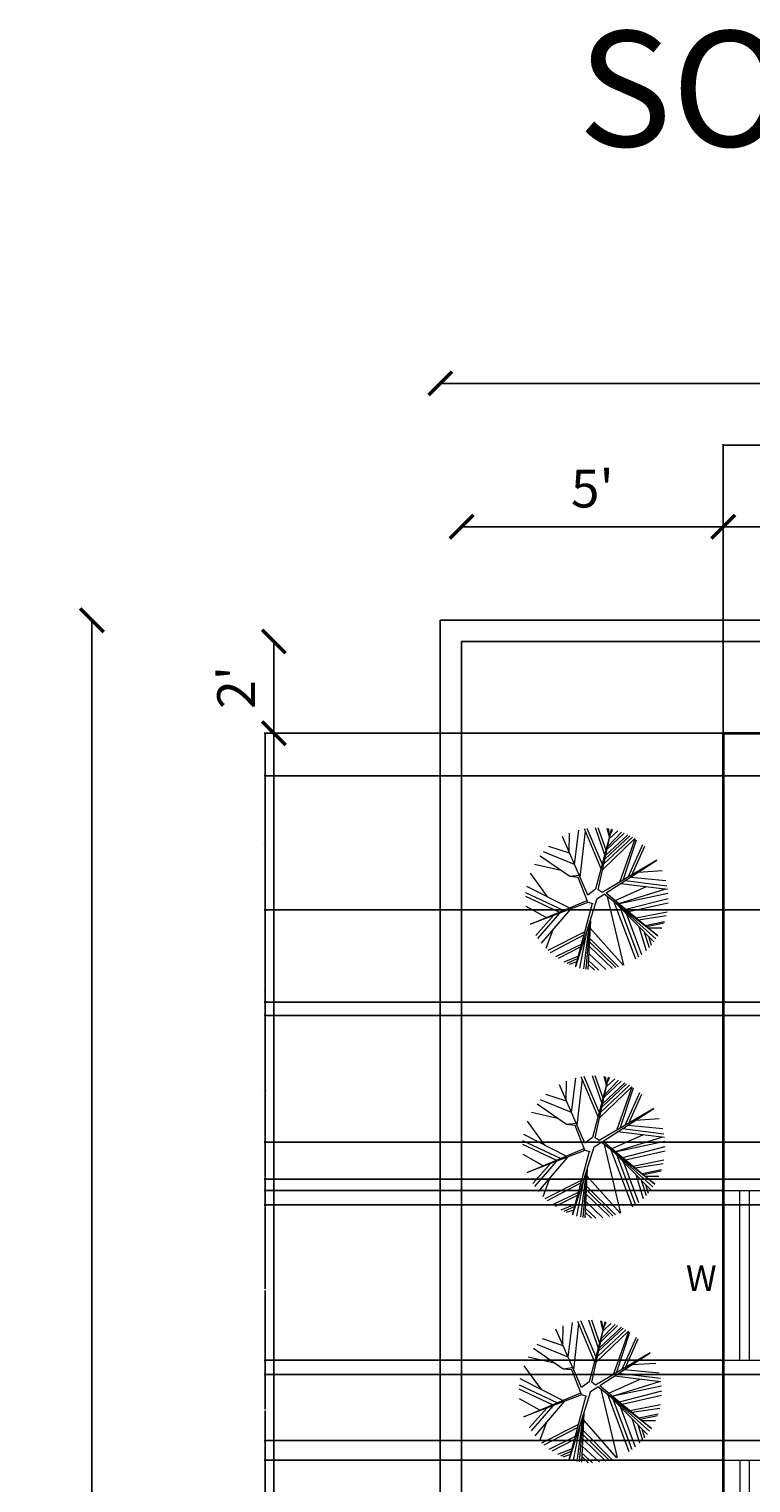
# Model space of a CAD drawing. Units: inches. Extents: x 503 to 1084, y -605 to 132.
# Tile 12 of 14: x 503 to 656, y -177 to 132. Entities that reach past the tile are written whole.
import ezdxf

# ---------------------------------------------------------------- set-up
doc = ezdxf.new("R2010")
doc.units = ezdxf.units.IN
doc.header["$MEASUREMENT"] = 0
for name, color, linetype, lineweight in [('A-ANNO-DIMS', 7, 'Continuous', 18), ('A-ANNO-TEXT', 7, 'Continuous', 18), ('C-PROP', 1, 'Continuous', 25), ('wall', 1, 'Continuous', 35), ('wind', 5, 'Continuous', 18)]:
    doc.layers.add(name, color=color, linetype=linetype, lineweight=lineweight)
doc.layers.add('GRASS', color=90, linetype='Continuous', lineweight=13, transparency=0.7)
doc.styles.get("Standard").update_dxf_attribs({"font": 'arial.ttf'})
doc.dimstyles.get("Standard").update_dxf_attribs({"dimtxt": 0.18, "dimasz": 0.18, "dimexe": 0.18, "dimexo": 0.0625, "dimgap": 0.09, "dimtad": 0, "dimtih": 1, "dimtoh": 1, "dimdec": 1, "dimzin": 0, "dimdsep": 46, "dimlunit": 4, "dimtxsty": 'Standard', "dimcen": 0.09, "dimadec": 0, "dimazin": 0, "dimtfac": 1, "dimtdec": 1, "dimtofl": 0, "dimtmove": 0, "dimatfit": 3, "dimfxl": 1, "dimtolj": 1, "dimtzin": 0, "dimarcsym": 0})

# ---------------------------------------------------------------- blocks, each defined once
blk = doc.blocks.new('A$C4FA53466')
at = {"color": 0}
for p, q in [((0.717, 0.864), (0.422, 1.538)), ((0.501, 1.356), (0.505, 1.578)), ((0.563, 1.216), (0.612, 1.614)), ((0.627, 1.07), (0.687, 1.601)), ((0.867, 1.166), (0.675, 1.628)), ((0.882, 1.223), (0.709, 1.633)), ((0.91, 1.328), (0.802, 1.64)), ((0.988, 1.623), (0.804, 0.931)), ((0.925, 1.384), (0.834, 1.64)), ((0.836, 0.927), (0.988, 1.623)), ((0.887, 1.159), (1.256, 1.515)), ((0.901, 1.223), (1.228, 1.532)), ((0.914, 1.283), (1.197, 1.549)), ((0.922, 1.323), (1.176, 1.559)), ((0.964, 1.534), (0.938, 1.632)), ((0.938, 1.393), (1.132, 1.579)), ((0.945, 1.425), (1.104, 1.59)), ((0.967, 1.545), (0.952, 1.63)), ((0.965, 1.517), (1.059, 1.605)), ((0.974, 1.559), (1.002, 1.62)), ((1.085, 1.015), (1.262, 1.512)), ((0.562, 1.217), (0.205, 1.363)), ((0.505, 1.347), (0.266, 1.426)), ((1.121, 1.036), (1.274, 1.503)), ((1.18, 1.071), (1.349, 1.447)), ((1.222, 1.096), (1.37, 1.428)), ((0.406, 1.148), (0.102, 1.217)), ((0.506, 1.079), (0.165, 1.314)), ((1.509, 1.265), (0.879, 0.894)), ((0.926, 0.889), (1.509, 1.265)), ((0.255, 0.841), (0.055, 1.116)), ((0.614, 1.092), (0.506, 1.079)), ((0.604, 1.069), (0.506, 1.079)), ((0.715, 0.784), (0.604, 1.069)), ((1.148, 1.032), (1.626, 0.972)), ((1.211, 1.073), (1.612, 1.034)), ((1.3, 1.13), (1.573, 1.147)), ((0.384, 0.667), (0, 0.848)), ((0.436, 0.689), (0.003, 0.892)), ((0.501, 0.716), (0.012, 0.965)), ((0.804, 0.931), (0.717, 0.864)), ((0.82, 0.82), (0.904, 0.875)), ((0.879, 0.894), (0.836, 0.927)), ((1.521, 0.394), (0.904, 0.875)), ((0.926, 0.889), (1.521, 0.394)), ((0.938, 0.848), (1.126, 0.059)), ((1.03, 0.802), (1.392, 0.963)), ((1.073, 0.767), (1.614, 0.936)), ((1.081, 0.769), (1.638, 0.886)), ((1.097, 0.999), (1.632, 0.934)), ((0.237, 0.605), (0.004, 0.735)), ((0.053, 0.528), (0.708, 0.803)), ((0.716, 0.781), (0.053, 0.528)), ((0.516, 0.704), (0.179, 0.309)), ((0.82, 0.82), (0.575, 0.037)), ((0.575, 0.037), (0.769, 0.772)), ((0.715, 0.784), (0.775, 0.767)), ((1.016, 0.788), (1.263, 0.13)), ((1.04, 0.769), (1.475, 0.326)), ((1.06, 0.754), (1.5, 0.362)), ((1.083, 0.725), (1.298, 0.153)), ((1.153, 0.701), (1.64, 0.826)), ((1.185, 0.674), (1.639, 0.776)), ((1.273, 0.601), (1.627, 0.672)), ((0.321, 0.63), (0.115, 0.4)), ((0.387, 0.655), (0.137, 0.366)), ((0.732, 0.539), (0.664, 0.015)), ((0.737, 0.554), (0.691, 0.01)), ((0.744, 0.569), (0.717, 0.006)), ((1.161, 0.646), (1.335, 0.182)), ((1.298, 0.58), (1.618, 0.629)), ((1.301, 0.503), (1.386, 0.227)), ((1.376, 0.515), (1.599, 0.562)), ((1.392, 0.502), (1.593, 0.545)), ((0.313, 0.466), (0.232, 0.248)), ((0.682, 0.44), (0.255, 0.225)), ((0.673, 0.407), (0.281, 0.201)), ((0.701, 0.44), (0.621, 0.024)), ((0.735, 0.369), (1.067, 0.038)), ((0.74, 0.488), (1.121, 0.057)), ((1.365, 0.438), (1.42, 0.26)), ((1.412, 0.486), (1.569, 0.486)), ((1.413, 0.39), (1.444, 0.288)), ((0.645, 0.301), (0.342, 0.153)), ((0.636, 0.267), (0.375, 0.133)), ((0.726, 0.192), (0.924, 0.006)), ((0.73, 0.277), (0.998, 0.019)), ((0.733, 0.326), (1.037, 0.029)), ((0.608, 0.161), (0.439, 0.093)), ((0.6, 0.133), (0.475, 0.076)), ((0.59, 0.094), (0.501, 0.064)), ((0.72, 0.07), (0.793, 0)), ((0.722, 0.111), (0.842, 0))]:
    blk.add_line(p, q, dxfattribs=at)
blk = doc.blocks.new('_ArchTick')
at = {"color": 0, "linetype": 'ByBlock', "const_width": 0.15}
blk.add_lwpolyline([(-0.5, -0.5), (0.5, 0.5)], dxfattribs=at)
blk = doc.blocks.new('*D5')
at = {"layer": 'A-ANNO-DIMS', "color": 0, "lineweight": -3, "transparency": 16777216}
blk.add_line((590.09, 56.42), (1046.09, 56.42), dxfattribs=at)
at = {"layer": 'Defpoints', "color": 0, "transparency": 16777216}
for p in [(1046.09, 56.42), (590.09, 6.18), (1046.09, 6.18)]:
    blk.add_point(p, dxfattribs=at)
at = {"layer": 'A-ANNO-DIMS', "color": 0, "lineweight": -3, "transparency": 16777216, "xscale": 5, "yscale": 5, "zscale": 5, "rotation": 180}
blk.add_blockref('_ArchTick', (590.09, 56.42), dxfattribs=at)
at = {"layer": 'A-ANNO-DIMS', "color": 0, "lineweight": -3, "transparency": 16777216, "xscale": 5, "yscale": 5, "zscale": 5}
blk.add_blockref('_ArchTick', (1046.09, 56.42), dxfattribs=at)
at = {"layer": 'A-ANNO-DIMS', "color": 0, "transparency": 16777216, "insert": (818.09, 64.51), "char_height": 8, "attachment_point": 5}
blk.add_mtext("\\A1;38'", dxfattribs=at)
blk = doc.blocks.new('*D6')
at = {"layer": 'A-ANNO-DIMS', "color": 0, "lineweight": -3, "transparency": 16777216}
blk.add_line((594.59, 26.02), (650.09, 26.02), dxfattribs=at)
at = {"layer": 'Defpoints', "color": 0, "transparency": 16777216}
for p in [(650.09, 26.02), (594.59, -17.82), (650.09, -17.82)]:
    blk.add_point(p, dxfattribs=at)
at = {"layer": 'A-ANNO-DIMS', "color": 0, "lineweight": -3, "transparency": 16777216, "xscale": 5, "yscale": 5, "zscale": 5, "rotation": 180}
blk.add_blockref('_ArchTick', (594.59, 26.02), dxfattribs=at)
at = {"layer": 'A-ANNO-DIMS', "color": 0, "lineweight": -3, "transparency": 16777216, "xscale": 5, "yscale": 5, "zscale": 5}
blk.add_blockref('_ArchTick', (650.09, 26.02), dxfattribs=at)
at = {"layer": 'A-ANNO-DIMS', "color": 0, "transparency": 16777216, "insert": (622.34, 34.09), "char_height": 8, "attachment_point": 5}
blk.add_mtext("\\A1;5'", dxfattribs=at)
blk = doc.blocks.new('*D7')
at = {"layer": 'A-ANNO-DIMS', "color": 0, "lineweight": -3, "transparency": 16777216}
blk.add_line((650.09, 26.02), (986.09, 26.02), dxfattribs=at)
at = {"layer": 'Defpoints', "color": 0, "transparency": 16777216}
for p in [(986.09, 26.02), (650.09, -17.82), (986.09, -17.82)]:
    blk.add_point(p, dxfattribs=at)
at = {"layer": 'A-ANNO-DIMS', "color": 0, "lineweight": -3, "transparency": 16777216, "xscale": 5, "yscale": 5, "zscale": 5, "rotation": 180}
blk.add_blockref('_ArchTick', (650.09, 26.02), dxfattribs=at)
at = {"layer": 'A-ANNO-DIMS', "color": 0, "lineweight": -3, "transparency": 16777216, "xscale": 5, "yscale": 5, "zscale": 5}
blk.add_blockref('_ArchTick', (986.09, 26.02), dxfattribs=at)
at = {"layer": 'A-ANNO-DIMS', "color": 0, "transparency": 16777216, "insert": (818.09, 34.1), "char_height": 8, "attachment_point": 5}
blk.add_mtext("\\A1;28'", dxfattribs=at)
blk = doc.blocks.new('_Oblique')
at = {"color": 0, "linetype": 'ByBlock', "lineweight": -2}
blk.add_line((-0.5, -0.5), (0.5, 0.5), dxfattribs=at)
blk = doc.blocks.new('*D10')
at = {"layer": 'A-ANNO-DIMS', "color": 0, "lineweight": -2, "transparency": 16777216}
blk.add_line((516.2, 6.18), (516.2, -545.82), dxfattribs=at)
at = {"layer": 'Defpoints', "color": 0, "transparency": 16777216}
for p in [(590.09, 6.18), (516.2, -545.82), (590.09, -545.82)]:
    blk.add_point(p, dxfattribs=at)
at = {"layer": 'A-ANNO-DIMS', "color": 0, "lineweight": -2, "transparency": 16777216, "xscale": 5, "yscale": 5, "zscale": 5}
for name, p, rotation in [('_ArchTick', (516.2, 6.18), 90), ('_Oblique', (516.2, -545.82), 270)]:
    blk.add_blockref(name, p, dxfattribs=dict(at, rotation=rotation))
at = {"layer": 'A-ANNO-DIMS', "color": 0, "transparency": 16777216, "insert": (508.12, -269.82), "char_height": 8, "attachment_point": 5, "rotation": 90}
blk.add_mtext("\\A1;46'", dxfattribs=at)
blk = doc.blocks.new('*D11')
at = {"layer": 'A-ANNO-DIMS', "color": 0, "lineweight": -2, "transparency": 16777216}
blk.add_line((554.79, 1.68), (554.79, -17.82), dxfattribs=at)
at = {"layer": 'Defpoints', "color": 0, "transparency": 16777216}
for p in [(650.94, 1.68), (554.79, -17.82), (650.09, -17.82)]:
    blk.add_point(p, dxfattribs=at)
at = {"layer": 'A-ANNO-DIMS', "color": 0, "lineweight": -2, "transparency": 16777216, "xscale": 5, "yscale": 5, "zscale": 5}
for name, p, rotation in [('_ArchTick', (554.79, 1.68), 90), ('_Oblique', (554.79, -17.82), 270)]:
    blk.add_blockref(name, p, dxfattribs=dict(at, rotation=rotation))
at = {"layer": 'A-ANNO-DIMS', "color": 0, "transparency": 16777216, "insert": (546.77, -8.07), "char_height": 8, "attachment_point": 5, "rotation": 90}
blk.add_mtext("\\A1;2'", dxfattribs=at)
blk = doc.blocks.new('*D12')
at = {"layer": 'A-ANNO-DIMS', "color": 0, "lineweight": -2, "transparency": 16777216}
blk.add_line((554.79, -17.82), (554.79, -442.82), dxfattribs=at)
at = {"layer": 'Defpoints', "color": 0, "transparency": 16777216}
for p in [(650.09, -17.82), (554.79, -442.82), (650.09, -442.82)]:
    blk.add_point(p, dxfattribs=at)
at = {"layer": 'A-ANNO-DIMS', "color": 0, "lineweight": -2, "transparency": 16777216, "xscale": 5, "yscale": 5, "zscale": 5}
for name, p, rotation in [('_ArchTick', (554.79, -17.82), 90), ('_Oblique', (554.79, -442.82), 270)]:
    blk.add_blockref(name, p, dxfattribs=dict(at, rotation=rotation))
at = {"layer": 'A-ANNO-DIMS', "color": 0, "transparency": 16777216, "insert": (546.7, -230.32), "char_height": 8, "attachment_point": 5, "rotation": 90}
blk.add_mtext("\\A1;36'", dxfattribs=at)
blk = doc.blocks.new('WIN-36IN')
for p, q in [((0, 0), (0, 9)), ((36, 0), (36, 9)), ((0, 5.5), (36, 5.5)), ((0, 3.5), (36, 3.5))]:
    blk.add_line(p, q)
blk = doc.blocks.new('VENT-24IN')
for p, q in [((0, 9), (0, 0)), ((24, 9), (24, 0)), ((24, 5.5), (0, 5.5)), ((24, 3.5), (0, 3.5))]:
    blk.add_line(p, q)
blk = doc.blocks.new('*D49')
at = {"layer": 'A-ANNO-DIMS', "color": 0, "lineweight": -2, "transparency": 16777216}
for p, q in [((650.09, -17.75), (650.09, 43.51)), ((650.27, 43.33), (676.21, 43.33)), ((702.82, 43.33), (676.88, 43.33)), ((703, -17.75), (703, 43.51))]:
    blk.add_line(p, q, dxfattribs=at)
at = {"layer": 'A-ANNO-DIMS', "color": 0, "transparency": 16777216}
for points in [[(650.27, 43.36), (650.27, 43.3), (650.09, 43.33)], [(702.82, 43.36), (702.82, 43.3), (703, 43.33)]]:
    blk.add_solid(points, dxfattribs=at)
at = {"layer": 'Defpoints', "color": 0, "transparency": 16777216}
for p in [(703, 43.33), (650.09, -17.82), (703, -17.82)]:
    blk.add_point(p, dxfattribs=at)
at = {"layer": 'A-ANNO-DIMS', "color": 0, "transparency": 16777216, "insert": (676.54, 43.33), "char_height": 0.18, "attachment_point": 5}
blk.add_mtext('\\A1;4\'-5"', dxfattribs=at)
blk = doc.blocks.new('*D52')
at = {"layer": 'A-ANNO-DIMS', "color": 0, "lineweight": -2, "transparency": 16777216}
for p, q in [((650.03, -17.82), (552.76, -17.82)), ((552.94, -18), (552.94, -66.11)), ((552.94, -114.59), (552.94, -66.48)), ((650.03, -114.77), (552.76, -114.77))]:
    blk.add_line(p, q, dxfattribs=at)
at = {"layer": 'A-ANNO-DIMS', "color": 0, "transparency": 16777216}
for points in [[(552.91, -18), (552.97, -18), (552.94, -17.82)], [(552.91, -114.59), (552.97, -114.59), (552.94, -114.77)]]:
    blk.add_solid(points, dxfattribs=at)
at = {"layer": 'Defpoints', "color": 0, "transparency": 16777216}
for p in [(650.09, -17.82), (552.94, -114.77), (650.09, -114.77)]:
    blk.add_point(p, dxfattribs=at)
at = {"layer": 'A-ANNO-DIMS', "color": 0, "transparency": 16777216, "insert": (552.94, -66.29), "char_height": 0.18, "attachment_point": 5}
blk.add_mtext('\\A1;8\'-1"', dxfattribs=at)
blk = doc.blocks.new('*D53')
at = {"layer": 'A-ANNO-DIMS', "color": 0, "lineweight": -2, "transparency": 16777216}
for p, q in [((650.03, -150.77), (552.76, -150.77)), ((552.94, -150.95), (552.94, -161.19)), ((552.94, -171.8), (552.94, -161.56)), ((650.03, -171.98), (552.76, -171.98))]:
    blk.add_line(p, q, dxfattribs=at)
at = {"layer": 'A-ANNO-DIMS', "color": 0, "transparency": 16777216}
for points in [[(552.91, -150.95), (552.97, -150.95), (552.94, -150.77)], [(552.91, -171.8), (552.97, -171.8), (552.94, -171.98)]]:
    blk.add_solid(points, dxfattribs=at)
at = {"layer": 'Defpoints', "color": 0, "transparency": 16777216}
for p in [(650.09, -150.77), (552.94, -171.98), (650.09, -171.98)]:
    blk.add_point(p, dxfattribs=at)
at = {"layer": 'A-ANNO-DIMS', "color": 0, "transparency": 16777216, "insert": (552.94, -161.38), "char_height": 0.18, "attachment_point": 5}
blk.add_mtext('\\A1;1\'-9"', dxfattribs=at)
blk = doc.blocks.new('*D56')
at = {"layer": 'A-ANNO-DIMS', "color": 0, "lineweight": -2, "transparency": 16777216}
for p, q in [((779.03, -167.82), (552.76, -167.82)), ((552.94, -168), (552.94, -185.63)), ((552.94, -203.64), (552.94, -186)), ((779.03, -203.82), (552.76, -203.82))]:
    blk.add_line(p, q, dxfattribs=at)
at = {"layer": 'A-ANNO-DIMS', "color": 0, "transparency": 16777216}
for points in [[(552.91, -168), (552.97, -168), (552.94, -167.82)], [(552.91, -203.64), (552.97, -203.64), (552.94, -203.82)]]:
    blk.add_solid(points, dxfattribs=at)
at = {"layer": 'Defpoints', "color": 0, "transparency": 16777216}
for p in [(779.09, -167.82), (552.94, -203.82), (779.09, -203.82)]:
    blk.add_point(p, dxfattribs=at)
at = {"layer": 'A-ANNO-DIMS', "color": 0, "transparency": 16777216, "insert": (552.94, -185.82), "char_height": 0.18, "attachment_point": 5}
blk.add_mtext('\\A1;3\'-0"', dxfattribs=at)
blk = doc.blocks.new('*D59')
at = {"layer": 'A-ANNO-DIMS', "color": 0, "lineweight": -2, "transparency": 16777216}
for p, q in [((779.03, -117.82), (552.76, -117.82)), ((552.94, -118), (552.94, -135.63)), ((552.94, -153.64), (552.94, -136)), ((779.03, -153.82), (552.76, -153.82))]:
    blk.add_line(p, q, dxfattribs=at)
at = {"layer": 'A-ANNO-DIMS', "color": 0, "transparency": 16777216}
for points in [[(552.91, -118), (552.97, -118), (552.94, -117.82)], [(552.91, -153.64), (552.97, -153.64), (552.94, -153.82)]]:
    blk.add_solid(points, dxfattribs=at)
at = {"layer": 'Defpoints', "color": 0, "transparency": 16777216}
for p in [(779.09, -117.82), (552.94, -153.82), (779.09, -153.82)]:
    blk.add_point(p, dxfattribs=at)
at = {"layer": 'A-ANNO-DIMS', "color": 0, "transparency": 16777216, "insert": (552.94, -135.82), "char_height": 0.18, "attachment_point": 5}
blk.add_mtext('\\A1;3\'-0"', dxfattribs=at)
blk = doc.blocks.new('*D61')
at = {"layer": 'A-ANNO-DIMS', "color": 0, "lineweight": -2, "transparency": 16777216}
for p, q in [((749.026202, -26.815853), (552.758702, -26.815853)), ((552.938702, -26.995853), (552.938702, -72.135853)), ((552.938702, -117.635853), (552.938702, -72.495853)), ((749.026202, -117.815853), (552.758702, -117.815853))]:
    blk.add_line(p, q, dxfattribs=at)
at = {"layer": 'A-ANNO-DIMS', "color": 0, "transparency": 16777216}
for points in [[(552.908702, -26.995853), (552.968702, -26.995853), (552.938702, -26.815853)], [(552.908702, -117.635853), (552.968702, -117.635853), (552.938702, -117.815853)]]:
    blk.add_solid(points, dxfattribs=at)
at = {"layer": 'Defpoints', "color": 0, "transparency": 16777216}
for p in [(552.938702, -26.815853), (749.088702, -26.815853), (749.088702, -117.815853)]:
    blk.add_point(p, dxfattribs=at)
at = {"layer": 'A-ANNO-DIMS', "color": 0, "transparency": 16777216, "insert": (552.938702, -72.315853), "char_height": 0.18, "attachment_point": 5}
blk.add_mtext('\\A1;7\'-7"', dxfattribs=at)
blk = doc.blocks.new('*D70')
at = {"layer": 'A-ANNO-DIMS', "color": 0, "lineweight": -2, "transparency": 16777216}
for p, q in [((817.28, -77.69), (552.76, -77.69)), ((552.94, -77.87), (552.94, -90.94)), ((552.94, -104.38), (552.94, -91.31)), ((817.28, -104.56), (552.76, -104.56))]:
    blk.add_line(p, q, dxfattribs=at)
at = {"layer": 'A-ANNO-DIMS', "color": 0, "transparency": 16777216}
for points in [[(552.91, -77.87), (552.97, -77.87), (552.94, -77.69)], [(552.91, -104.38), (552.97, -104.38), (552.94, -104.56)]]:
    blk.add_solid(points, dxfattribs=at)
at = {"layer": 'Defpoints', "color": 0, "transparency": 16777216}
for p in [(817.34, -77.69), (552.94, -104.56), (817.34, -104.56)]:
    blk.add_point(p, dxfattribs=at)
at = {"layer": 'A-ANNO-DIMS', "color": 0, "transparency": 16777216, "insert": (552.94, -91.12), "char_height": 0.18, "attachment_point": 5}
blk.add_mtext('\\A1;2\'-3"', dxfattribs=at)
blk = doc.blocks.new('*D74')
at = {"layer": 'A-ANNO-DIMS', "color": 0, "lineweight": -2, "transparency": 16777216}
for p, q in [((751.01, -74.83), (552.76, -74.83)), ((552.94, -75.01), (552.94, -93.43)), ((552.94, -112.21), (552.94, -93.8)), ((751.01, -112.39), (552.76, -112.39))]:
    blk.add_line(p, q, dxfattribs=at)
at = {"layer": 'A-ANNO-DIMS', "color": 0, "transparency": 16777216}
for points in [[(552.91, -75.01), (552.97, -75.01), (552.94, -74.83)], [(552.91, -112.21), (552.97, -112.21), (552.94, -112.39)]]:
    blk.add_solid(points, dxfattribs=at)
at = {"layer": 'Defpoints', "color": 0, "transparency": 16777216}
for p in [(751.07, -74.83), (552.94, -112.39), (751.07, -112.39)]:
    blk.add_point(p, dxfattribs=at)
at = {"layer": 'A-ANNO-DIMS', "color": 0, "transparency": 16777216, "insert": (552.94, -93.61), "char_height": 0.18, "attachment_point": 5}
blk.add_mtext('\\A1;3\'-1 1/2"', dxfattribs=at)
blk = doc.blocks.new('*D75')
at = {"layer": 'A-ANNO-DIMS', "color": 0, "lineweight": -2, "transparency": 16777216}
for p, q in [((749.03, -26.82), (552.76, -26.82)), ((552.94, -27), (552.94, -40.85)), ((552.94, -55.08), (552.94, -41.22)), ((749.03, -55.26), (552.76, -55.26))]:
    blk.add_line(p, q, dxfattribs=at)
at = {"layer": 'A-ANNO-DIMS', "color": 0, "transparency": 16777216}
for points in [[(552.91, -27), (552.97, -27), (552.94, -26.82)], [(552.91, -55.08), (552.97, -55.08), (552.94, -55.26)]]:
    blk.add_solid(points, dxfattribs=at)
at = {"layer": 'Defpoints', "color": 0, "transparency": 16777216}
for p in [(749.09, -26.82), (552.94, -55.26), (749.09, -55.26)]:
    blk.add_point(p, dxfattribs=at)
at = {"layer": 'A-ANNO-DIMS', "color": 0, "transparency": 16777216, "insert": (552.94, -41.04), "char_height": 0.18, "attachment_point": 5}
blk.add_mtext('\\A1;2\'-4 1/2"', dxfattribs=at)

msp = doc.modelspace()

# ---------------------------------------------------------------- linework, layer by layer
at = {"layer": 'C-PROP'}
for p, q in [((590.09, 6.18), (590.09, -545.82)), ((590.09, 6.18), (1046.09, 6.18)), ((1041.59, 1.68), (594.59, 1.68)), ((594.59, -541.32), (594.59, 1.68))]:
    msp.add_line(p, q, dxfattribs=at)
at = {"layer": 'wall'}
for q in [(986.09, -17.82), (650.09, -514.82)]:
    msp.add_line((650.09, -17.82), q, dxfattribs=at)

# ---------------------------------------------------------------- block references
at = {"layer": 'GRASS', "xscale": 18.41745235960633, "yscale": 18.41745235960633, "zscale": 18.41745235960633}
for p in [(608.21, -68.06), (607.57, -120.68), (606.84, -172.54)]:
    msp.add_blockref('A$C4FA53466', p, dxfattribs=at)
at = {"layer": 'wind'}
for name, p, rotation in [('WIN-36IN', (650.08, -114.78), 270), ('VENT-24IN', (659.09, -195.98), 90.00000000000081)]:
    msp.add_blockref(name, p, dxfattribs=dict(at, rotation=rotation))

# ---------------------------------------------------------------- texts
at = {"layer": 'A-ANNO-TEXT'}
msp.add_text('W', height=5.44, dxfattribs=at).set_placement((642.19, -136.1))
at = {"layer": 'A-ANNO-TEXT', "insert": (619.28, 131.14), "char_height": 24.4528, "attachment_point": 1}
msp.add_mtext_dynamic_manual_height_columns('SOUTH FACING HOUSE', width=395.3147, gutter_width=4.08, heights=[0], dxfattribs=at)

# ---------------------------------------------------------------- dimensions: what is measured, and where the dimension line sits
at = {"layer": 'A-ANNO-DIMS'}
for base, p1, p2, override, picture, middle in [((1046.09, 56.42), (590.09, 6.18), (1046.09, 6.18), {"dimtxt": 8, "dimasz": 5, "dimgap": 4, "dimtad": 1, "dimblk1": 'ArchTick', "dimblk2": 'ArchTick', "dimsah": 1, "dimse1": 1, "dimse2": 1, "dimclrd": 0, "dimclre": 0, "dimclrt": 0, "dimlwd": -3}, '*D5', (818.09, 64.51)), ((703, 43.33), (650.09, -17.82), (703, -17.82), {"dimdec": 1, "dimlfac": 1, "dimrnd": 0, "dimzin": 1, "dimdsep": 46, "dimlunit": 4, "dimfrac": 2}, '*D49', (676.54, 43.33)), ((986.09, 26.02), (650.09, -17.82), (986.09, -17.82), {"dimtxt": 8, "dimasz": 5, "dimgap": 4, "dimtad": 1, "dimblk1": 'ArchTick', "dimblk2": 'ArchTick', "dimsah": 1, "dimse1": 1, "dimse2": 1, "dimclrd": 0, "dimclre": 0, "dimclrt": 0, "dimlwd": -3}, '*D7', (818.09, 34.1))]:
    dim = msp.add_linear_dim(base=base, p1=p1, p2=p2, dimstyle='Standard', override=override, dxfattribs=at)
    dim.commit()
    dim.dimension.update_dxf_attribs({"geometry": picture, "text_midpoint": middle})
dim = msp.add_linear_dim(base=(650.09, 26.02), p1=(594.59, -17.82), p2=(650.09, -17.82), text="5'", dimstyle='Standard', override={"dimtxt": 8, "dimasz": 5, "dimgap": 4, "dimtad": 1, "dimblk1": 'ArchTick', "dimblk2": 'ArchTick', "dimsah": 1, "dimse1": 1, "dimse2": 1, "dimclrd": 0, "dimclre": 0, "dimclrt": 0, "dimlwd": -3}, dxfattribs=at)
dim.commit()
dim.dimension.update_dxf_attribs({"geometry": '*D6', "text_midpoint": (622.34, 34.09)})
for base, p1, p2, override, picture, middle in [((516.2, -545.82), (590.09, 6.18), (590.09, -545.82), {"dimtxt": 8, "dimasz": 5, "dimgap": 4, "dimtad": 1, "dimtih": 0, "dimblk1": 'ArchTick', "dimblk2": 'Oblique', "dimsah": 1, "dimse1": 1, "dimse2": 1, "dimclrd": 0, "dimclre": 0, "dimclrt": 0}, '*D10', (508.12, -269.82)), ((552.9387, -114.772), (650.0887, -17.8159), (650.0887, -114.772), {"dimdec": 1, "dimlfac": 1, "dimrnd": 0, "dimzin": 1, "dimdsep": 46, "dimlunit": 4, "dimfrac": 2}, '*D52', (552.9387, -66.2939)), ((552.94, -55.26), (749.09, -26.82), (749.09, -55.26), {"dimdec": 1, "dimlfac": 1, "dimrnd": 0, "dimzin": 1, "dimdsep": 46, "dimlunit": 4, "dimfrac": 2}, '*D75', (552.94, -41.04)), ((552.94, -26.82), (749.09, -117.82), (749.09, -26.82), {"dimdec": 1, "dimlfac": 1, "dimrnd": 0, "dimzin": 1, "dimdsep": 46, "dimlunit": 4, "dimfrac": 2}, '*D61', (552.94, -72.32)), ((552.94, -112.39), (751.07, -74.83), (751.07, -112.39), {"dimdec": 1, "dimlfac": 1, "dimrnd": 0, "dimzin": 1, "dimdsep": 46, "dimlunit": 4, "dimfrac": 2}, '*D74', (552.94, -93.61)), ((552.94, -104.56), (817.34, -77.69), (817.34, -104.56), {"dimdec": 1, "dimlfac": 1, "dimrnd": 0, "dimzin": 1, "dimdsep": 46, "dimlunit": 4, "dimfrac": 2}, '*D70', (552.94, -91.12)), ((552.94, -153.82), (779.09, -117.82), (779.09, -153.82), {"dimdec": 1, "dimlfac": 1, "dimrnd": 0, "dimzin": 1, "dimdsep": 46, "dimlunit": 4, "dimfrac": 2}, '*D59', (552.94, -135.82)), ((552.94, -171.98), (650.09, -150.77), (650.09, -171.98), {"dimdec": 1, "dimlfac": 1, "dimrnd": 0, "dimzin": 1, "dimdsep": 46, "dimlunit": 4, "dimfrac": 2}, '*D53', (552.94, -161.38)), ((552.94, -203.82), (779.09, -167.82), (779.09, -203.82), {"dimdec": 1, "dimlfac": 1, "dimrnd": 0, "dimzin": 1, "dimdsep": 46, "dimlunit": 4, "dimfrac": 2}, '*D56', (552.94, -185.82))]:
    dim = msp.add_linear_dim(base=base, p1=p1, p2=p2, angle=90, dimstyle='Standard', override=override, dxfattribs=at)
    dim.commit()
    dim.dimension.update_dxf_attribs({"geometry": picture, "text_midpoint": middle})
for base, p1, p2, text, picture, middle in [((554.79, -17.82), (650.94, 1.68), (650.09, -17.82), "2'", '*D11', (546.77, -8.07)), ((554.79, -442.82), (650.09, -17.82), (650.09, -442.82), "36'", '*D12', (546.7, -230.32))]:
    dim = msp.add_linear_dim(base=base, p1=p1, p2=p2, angle=90, text=text, dimstyle='Standard', override={"dimtxt": 8, "dimasz": 5, "dimgap": 4, "dimtad": 1, "dimtih": 0, "dimblk1": 'ArchTick', "dimblk2": 'Oblique', "dimsah": 1, "dimse1": 1, "dimse2": 1, "dimclrd": 0, "dimclre": 0, "dimclrt": 0}, dxfattribs=at)
    dim.commit()
    dim.dimension.update_dxf_attribs({"geometry": picture, "text_midpoint": middle})

doc.saveas('drawing.dxf')
